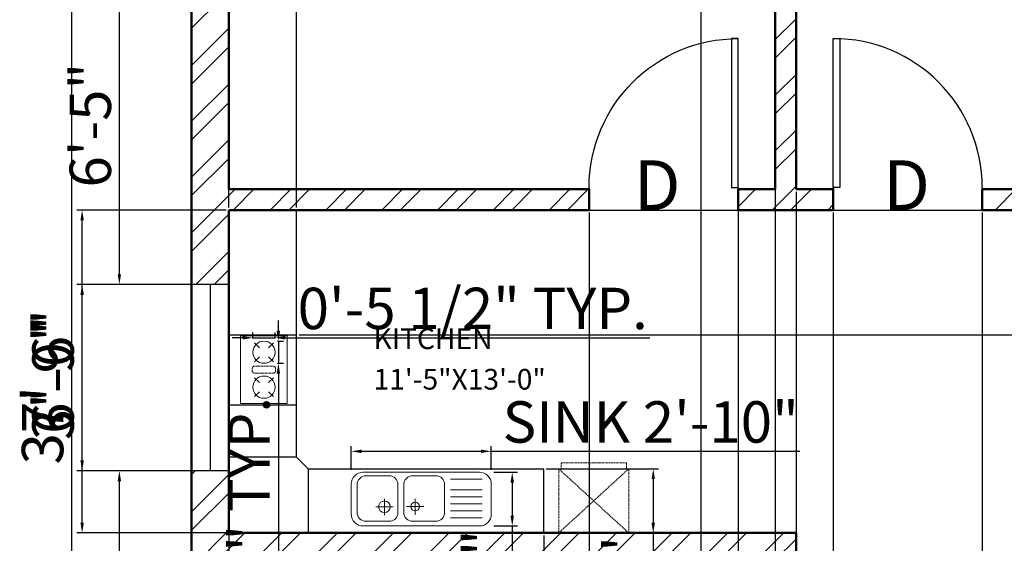
# Model space of a CAD drawing. Units: inches. Extents: x 3824 to 4289, y 1731 to 2259.
# Tile 3 of 5: x 3831 to 4069, y 1952 to 2079. Entities that reach past the tile are written whole.
import ezdxf

# ---------------------------------------------------------------- set-up
doc = ezdxf.new("R2010")
doc.units = ezdxf.units.IN
doc.linetypes.add('HIDDEN', pattern=[0.375, 0.25, -0.125])
for name, color, linetype, lineweight in [('A-ANNO-DIMS', 2, 'Continuous', 18), ('A-ANNO-TEXT', 2, 'Continuous', 18), ('A-AREA-IDEN', 2, 'Continuous', 18), ('A-EQPM', 9, 'Continuous', 18), ('A-EQPM-HIDN', 9, 'HIDDEN', 18), ('A-FLOR-CASE', 8, 'Continuous', 25), ('A-FLOR-FIXT', 9, 'Continuous', 18), ('A-FLOR-THRS', 8, 'Continuous', 18), ('DOOR', 6, 'Continuous', 25), ('WALL', 20, 'Continuous', 50), ('WINDOW', 4, 'Continuous', 25)]:
    doc.layers.add(name, color=color, linetype=linetype, lineweight=lineweight)
doc.layers.add('A-WALL-PATT', color=251, linetype='Continuous', lineweight=13, true_color=0x636466)
doc.styles.get("Standard").update_dxf_attribs({"font": 'arial.ttf'})
doc.dimstyles.new('ISO-25', dxfattribs={"dimtxt": 10, "dimasz": 2.5, "dimexe": 1.25, "dimexo": 0.625, "dimtad": 1, "dimdec": 1, "dimlunit": 3, "dimtxsty": 'Standard', "dimcen": 2.5, "dimadec": 0, "dimazin": 0, "dimtfac": 1, "dimtdec": 1, "dimtmove": 0, "dimatfit": 3, "dimfxl": 1, "dimarcsym": 0})

# ---------------------------------------------------------------- blocks, each defined once
blk = doc.blocks.new('*U2')
for p, q in [((0, 0), (0, -6)), ((40, 0), (40, -6))]:
    blk.add_line(p, q)
blk.add_lwpolyline([(0, 0), (0, 40), (1.75, 40), (1.75, 0)], close=True)
blk.add_arc((0, 0), 40, 0, 90)
blk = doc.blocks.new('SINK12RS')
for p, q in [((283, -292), (283, -153)), ((546, -293), (546, -154)), ((849, -130), (1120, -130)), ((209, -225), (359, -225)), ((472, -226), (622, -226)), ((849, -190), (1120, -190)), ((849, -250), (1120, -250)), ((849, -310), (1120, -310)), ((849, -370), (1120, -370)), ((849, -460), (1120, -460))]:
    blk.add_line(p, q)
for points in [[(99, -520), (1099, -520, 0.414214), (1199, -420), (1199, -160, 0.414214), (1099, -60), (99, -60, 0.414214), (-1, -160), (-1, -420, 0.414214)], [(124, -490), (324, -490, 0.414214), (399, -415), (399, -175, 0.414214), (324, -100), (124, -100, 0.414214), (49, -175), (49, -415, 0.414214)], [(524, -490, -0.414214), (449, -415), (449, -175, -0.414214), (524, -100), (724, -100, -0.414214), (799, -175), (799, -415, -0.414214), (724, -490)]]:
    blk.add_lwpolyline(points, format="xyb", close=True)
for centre, radius in [((283, -225), 50), ((546, -226), 37.5)]:
    blk.add_circle(centre, radius)
blk = doc.blocks.new('*D12')
at = {"layer": 'A-ANNO-DIMS', "color": 0, "lineweight": -2, "transparency": 16777216}
for p, q in [((3871.93, 2202.62), (3842.32, 2202.62)), ((3843.57, 2200.12), (3843.57, 1761.12)), ((3871.93, 1758.62), (3842.32, 1758.62))]:
    blk.add_line(p, q, dxfattribs=at)
at = {"layer": 'A-ANNO-DIMS', "color": 0, "transparency": 16777216}
for points in [[(3843.15, 2200.12), (3843.99, 2200.12), (3843.57, 2202.62)], [(3843.15, 1761.12), (3843.99, 1761.12), (3843.57, 1758.62)]]:
    blk.add_solid(points, dxfattribs=at)
at = {"layer": 'Defpoints', "color": 0, "transparency": 16777216}
for p in [(3872.55, 2202.62), (3843.57, 1758.62), (3872.55, 1758.62)]:
    blk.add_point(p, dxfattribs=at)
at = {"layer": 'A-ANNO-DIMS', "color": 0, "transparency": 16777216, "insert": (3837.84, 1980.62), "char_height": 10, "attachment_point": 5, "rotation": 90}
blk.add_mtext("37'", dxfattribs=at)
blk = doc.blocks.new('COOKTOP-BURNER')
for p, q in [((0.39, 4.97), (1.58, 3.77)), ((4.97, 4.97), (3.77, 3.77)), ((1.58, 1.58), (0.39, 0.39)), ((3.77, 1.58), (4.97, 0.39))]:
    blk.add_line(p, q)
blk.add_circle((2.68, 2.68), 2.68)
blk = doc.blocks.new('*D18')
at = {"layer": 'A-ANNO-DIMS', "color": 0, "lineweight": -2, "transparency": 16777216}
for p, q in [((3893.51, 2003.46), (3893.51, 2005.96)), ((3893.33, 2000.96), (3894.76, 2000.96)), ((3893.51, 2000.96), (3893.51, 1995.6)), ((3893.33, 1995.6), (3894.76, 1995.6)), ((3893.51, 1993.1), (3893.51, 1842.67))]:
    blk.add_line(p, q, dxfattribs=at)
at = {"layer": 'A-ANNO-DIMS', "color": 0, "transparency": 16777216}
for points in [[(3893.09, 2003.46), (3893.93, 2003.46), (3893.51, 2000.96)], [(3893.09, 1993.1), (3893.93, 1993.1), (3893.51, 1995.6)]]:
    blk.add_solid(points, dxfattribs=at)
at = {"layer": 'Defpoints', "color": 0, "transparency": 16777216}
for p in [(3892.71, 2000.96), (3892.71, 1995.6), (3893.51, 1995.6)]:
    blk.add_point(p, dxfattribs=at)
at = {"layer": 'A-ANNO-DIMS', "color": 0, "transparency": 16777216, "insert": (3887.71, 1916.64), "char_height": 10, "attachment_point": 5, "rotation": 90}
blk.add_mtext('BURNER 0\'-5 1/2" TYP.', dxfattribs=at)
blk = doc.blocks.new('*D19')
at = {"layer": 'A-ANNO-DIMS', "color": 0, "lineweight": -2, "transparency": 16777216}
for p, q in [((3887.35, 2001.58), (3887.35, 2003.01)), ((3892.71, 2001.58), (3892.71, 2003.01)), ((3884.85, 2001.76), (3882.35, 2001.76)), ((3887.35, 2001.76), (3892.71, 2001.76)), ((3895.21, 2001.76), (3983.21, 2001.76))]:
    blk.add_line(p, q, dxfattribs=at)
at = {"layer": 'A-ANNO-DIMS', "color": 0, "transparency": 16777216}
for points in [[(3884.85, 2002.17), (3884.85, 2001.34), (3887.35, 2001.76)], [(3895.21, 2002.17), (3895.21, 2001.34), (3892.71, 2001.76)]]:
    blk.add_solid(points, dxfattribs=at)
at = {"layer": 'Defpoints', "color": 0, "transparency": 16777216}
for p in [(3887.35, 2000.96), (3892.71, 2001.76), (3892.71, 2000.96)]:
    blk.add_point(p, dxfattribs=at)
at = {"layer": 'A-ANNO-DIMS', "color": 0, "transparency": 16777216, "insert": (3940.46, 2007.55), "char_height": 10, "attachment_point": 5}
blk.add_mtext('0\'-5 1/2" TYP.', dxfattribs=at)
blk = doc.blocks.new('*D22')
at = {"layer": 'A-ANNO-DIMS', "color": 0, "lineweight": -2, "transparency": 16777216}
for p, q in [((3911.13, 1969.89), (3911.13, 1975.59)), ((3913.63, 1974.34), (3942.43, 1974.34)), ((3944.93, 1969.89), (3944.93, 1975.59)), ((3944.93, 1974.34), (4019.47, 1974.34))]:
    blk.add_line(p, q, dxfattribs=at)
at = {"layer": 'A-ANNO-DIMS', "color": 0, "transparency": 16777216}
for points in [[(3913.63, 1974.75), (3913.63, 1973.92), (3911.13, 1974.34)], [(3942.43, 1974.75), (3942.43, 1973.92), (3944.93, 1974.34)]]:
    blk.add_solid(points, dxfattribs=at)
at = {"layer": 'Defpoints', "color": 0, "transparency": 16777216}
for p in [(3944.93, 1974.34), (3911.13, 1969.27), (3944.93, 1969.27)]:
    blk.add_point(p, dxfattribs=at)
at = {"layer": 'A-ANNO-DIMS', "color": 0, "transparency": 16777216, "insert": (3983.45, 1980.13), "char_height": 10, "attachment_point": 5}
blk.add_mtext('SINK 2\'-10"', dxfattribs=at)
blk = doc.blocks.new('*D23')
at = {"layer": 'A-ANNO-DIMS', "color": 0, "lineweight": -2, "transparency": 16777216}
for p, q in [((3945.56, 1969.27), (3951.25, 1969.27)), ((3950, 1966.77), (3950, 1958.81)), ((3945.56, 1956.31), (3951.25, 1956.31)), ((3950, 1956.31), (3950, 1926.92))]:
    blk.add_line(p, q, dxfattribs=at)
at = {"layer": 'A-ANNO-DIMS', "color": 0, "transparency": 16777216}
for points in [[(3949.58, 1966.77), (3950.42, 1966.77), (3950, 1969.27)], [(3949.58, 1958.81), (3950.42, 1958.81), (3950, 1956.31)]]:
    blk.add_solid(points, dxfattribs=at)
at = {"layer": 'Defpoints', "color": 0, "transparency": 16777216}
for p in [(3944.93, 1969.27), (3944.93, 1956.31), (3950, 1956.31)]:
    blk.add_point(p, dxfattribs=at)
at = {"layer": 'A-ANNO-DIMS', "color": 0, "transparency": 16777216, "insert": (3944.36, 1940.36), "char_height": 10, "attachment_point": 5, "rotation": 90}
blk.add_mtext('1\'-1"', dxfattribs=at)
blk = doc.blocks.new('*D28')
at = {"layer": 'A-ANNO-DIMS', "color": 0, "lineweight": -2, "transparency": 16777216}
for p, q in [((3880.93, 1969.62), (3853.85, 1969.62)), ((3855.1, 1904.12), (3855.1, 1967.12)), ((3880.93, 1901.62), (3853.85, 1901.62))]:
    blk.add_line(p, q, dxfattribs=at)
at = {"layer": 'A-ANNO-DIMS', "color": 0, "transparency": 16777216}
for points in [[(3854.69, 1967.12), (3855.52, 1967.12), (3855.1, 1969.62)], [(3854.69, 1904.12), (3855.52, 1904.12), (3855.1, 1901.62)]]:
    blk.add_solid(points, dxfattribs=at)
at = {"layer": 'Defpoints', "color": 0, "transparency": 16777216}
for p in [(3855.1, 1969.62), (3881.55, 1969.62), (3881.55, 1901.62)]:
    blk.add_point(p, dxfattribs=at)
at = {"layer": 'A-ANNO-DIMS', "color": 0, "transparency": 16777216, "insert": (3849.37, 1935.62), "char_height": 10, "attachment_point": 5, "rotation": 90}
blk.add_mtext('5\'-8"', dxfattribs=at)
blk = doc.blocks.new('*D29')
at = {"layer": 'A-ANNO-DIMS', "color": 0, "lineweight": -2, "transparency": 16777216}
for p, q in [((3871.93, 2014.62), (3844.85, 2014.62)), ((3846.1, 1972.12), (3846.1, 2012.12)), ((3871.93, 1969.62), (3844.85, 1969.62))]:
    blk.add_line(p, q, dxfattribs=at)
at = {"layer": 'A-ANNO-DIMS', "color": 0, "transparency": 16777216}
for points in [[(3845.69, 2012.12), (3846.52, 2012.12), (3846.1, 2014.62)], [(3845.69, 1972.12), (3846.52, 1972.12), (3846.1, 1969.62)]]:
    blk.add_solid(points, dxfattribs=at)
at = {"layer": 'Defpoints', "color": 0, "transparency": 16777216}
for p in [(3846.1, 2014.62), (3872.55, 2014.62), (3872.55, 1969.62)]:
    blk.add_point(p, dxfattribs=at)
at = {"layer": 'A-ANNO-DIMS', "color": 0, "transparency": 16777216, "insert": (3840.37, 1992.12), "char_height": 10, "attachment_point": 5, "rotation": 90}
blk.add_mtext('3\'-9"', dxfattribs=at)
blk = doc.blocks.new('*D30')
at = {"layer": 'A-ANNO-DIMS', "color": 0, "lineweight": -2, "transparency": 16777216}
for p, q in [((3880.93, 2091.62), (3853.85, 2091.62)), ((3855.1, 2017.12), (3855.1, 2089.12)), ((3880.93, 2014.62), (3853.85, 2014.62))]:
    blk.add_line(p, q, dxfattribs=at)
at = {"layer": 'A-ANNO-DIMS', "color": 0, "transparency": 16777216}
for points in [[(3854.69, 2089.12), (3855.52, 2089.12), (3855.1, 2091.62)], [(3854.69, 2017.12), (3855.52, 2017.12), (3855.1, 2014.62)]]:
    blk.add_solid(points, dxfattribs=at)
at = {"layer": 'Defpoints', "color": 0, "transparency": 16777216}
for p in [(3855.1, 2091.62), (3881.55, 2091.62), (3881.55, 2014.62)]:
    blk.add_point(p, dxfattribs=at)
at = {"layer": 'A-ANNO-DIMS', "color": 0, "transparency": 16777216, "insert": (3849.37, 2053.12), "char_height": 10, "attachment_point": 5, "rotation": 90}
blk.add_mtext('6\'-5"', dxfattribs=at)
blk = doc.blocks.new('*D42')
at = {"layer": 'A-ANNO-DIMS', "color": 0, "lineweight": -2, "transparency": 16777216}
for p, q in [((4004.55, 2036.99), (4004.55, 1730.92)), ((3968.55, 2031.99), (3968.55, 1730.92)), ((3971.05, 1732.17), (4002.05, 1732.17))]:
    blk.add_line(p, q, dxfattribs=at)
at = {"layer": 'A-ANNO-DIMS', "color": 0, "transparency": 16777216}
for points in [[(3971.05, 1732.59), (3971.05, 1731.75), (3968.55, 1732.17)], [(4002.05, 1732.59), (4002.05, 1731.75), (4004.55, 1732.17)]]:
    blk.add_solid(points, dxfattribs=at)
at = {"layer": 'Defpoints', "color": 0, "transparency": 16777216}
for p in [(4004.55, 2037.62), (3968.55, 2032.62), (4004.55, 1732.17)]:
    blk.add_point(p, dxfattribs=at)
at = {"layer": 'A-ANNO-DIMS', "color": 0, "transparency": 16777216, "insert": (3986.55, 1737.9), "char_height": 10, "attachment_point": 5}
blk.add_mtext('3\'-0"', dxfattribs=at)
blk = doc.blocks.new('*D43')
at = {"layer": 'A-ANNO-DIMS', "color": 0, "lineweight": -2, "transparency": 16777216}
for p, q in [((4004.55, 2036.99), (4004.55, 1730.92)), ((4013.55, 2036.99), (4013.55, 1730.92)), ((4007.05, 1732.17), (4011.05, 1732.17)), ((4013.55, 1732.17), (4043.88, 1732.17))]:
    blk.add_line(p, q, dxfattribs=at)
at = {"layer": 'A-ANNO-DIMS', "color": 0, "transparency": 16777216}
for points in [[(4007.05, 1732.59), (4007.05, 1731.75), (4004.55, 1732.17)], [(4011.05, 1732.59), (4011.05, 1731.75), (4013.55, 1732.17)]]:
    blk.add_solid(points, dxfattribs=at)
at = {"layer": 'Defpoints', "color": 0, "transparency": 16777216}
for p in [(4004.55, 2037.62), (4013.55, 2037.62), (4013.55, 1732.17)]:
    blk.add_point(p, dxfattribs=at)
at = {"layer": 'A-ANNO-DIMS', "color": 0, "transparency": 16777216, "insert": (4029.97, 1737.9), "char_height": 10, "attachment_point": 5}
blk.add_mtext('0\'-9"', dxfattribs=at)
blk = doc.blocks.new('*D44')
at = {"layer": 'A-ANNO-DIMS', "color": 0, "lineweight": -2, "transparency": 16777216}
for p, q in [((4018.55, 2036.99), (4018.55, 1730.92)), ((4027.55, 2031.99), (4027.55, 1730.92)), ((4021.05, 1732.17), (4025.05, 1732.17)), ((4027.55, 1732.17), (4057.88, 1732.17))]:
    blk.add_line(p, q, dxfattribs=at)
at = {"layer": 'A-ANNO-DIMS', "color": 0, "transparency": 16777216}
for points in [[(4021.05, 1732.59), (4021.05, 1731.75), (4018.55, 1732.17)], [(4025.05, 1732.59), (4025.05, 1731.75), (4027.55, 1732.17)]]:
    blk.add_solid(points, dxfattribs=at)
at = {"layer": 'Defpoints', "color": 0, "transparency": 16777216}
for p in [(4018.55, 2037.62), (4027.55, 2032.62), (4027.55, 1732.17)]:
    blk.add_point(p, dxfattribs=at)
at = {"layer": 'A-ANNO-DIMS', "color": 0, "transparency": 16777216, "insert": (4043.97, 1737.9), "char_height": 10, "attachment_point": 5}
blk.add_mtext('0\'-9"', dxfattribs=at)
blk = doc.blocks.new('*D45')
at = {"layer": 'A-ANNO-DIMS', "color": 0, "lineweight": -2, "transparency": 16777216}
for p, q in [((4027.55, 2031.99), (4027.55, 1730.92)), ((4063.55, 2031.99), (4063.55, 1730.92)), ((4030.05, 1732.17), (4061.05, 1732.17))]:
    blk.add_line(p, q, dxfattribs=at)
at = {"layer": 'A-ANNO-DIMS', "color": 0, "transparency": 16777216}
for points in [[(4030.05, 1732.59), (4030.05, 1731.75), (4027.55, 1732.17)], [(4061.05, 1732.59), (4061.05, 1731.75), (4063.55, 1732.17)]]:
    blk.add_solid(points, dxfattribs=at)
at = {"layer": 'Defpoints', "color": 0, "transparency": 16777216}
for p in [(4027.55, 2032.62), (4063.55, 2032.62), (4063.55, 1732.17)]:
    blk.add_point(p, dxfattribs=at)
at = {"layer": 'A-ANNO-DIMS', "color": 0, "transparency": 16777216, "insert": (4045.55, 1737.9), "char_height": 10, "attachment_point": 5}
blk.add_mtext('3\'-0"', dxfattribs=at)
blk = doc.blocks.new('*D56')
at = {"layer": 'A-ANNO-DIMS', "color": 0, "lineweight": -2, "transparency": 16777216}
for p, q in [((3995.55, 2120.99), (3995.55, 1730.92)), ((4013.55, 2120.99), (4013.55, 1730.92)), ((3998.05, 1732.17), (4011.05, 1732.17)), ((4013.55, 1732.17), (4042.94, 1732.17))]:
    blk.add_line(p, q, dxfattribs=at)
at = {"layer": 'A-ANNO-DIMS', "color": 0, "transparency": 16777216}
for points in [[(3998.05, 1732.59), (3998.05, 1731.75), (3995.55, 1732.17)], [(4011.05, 1732.59), (4011.05, 1731.75), (4013.55, 1732.17)]]:
    blk.add_solid(points, dxfattribs=at)
at = {"layer": 'Defpoints', "color": 0, "transparency": 16777216}
for p in [(3995.55, 2121.62), (4013.55, 2121.62), (4013.55, 1732.17)]:
    blk.add_point(p, dxfattribs=at)
at = {"layer": 'A-ANNO-DIMS', "color": 0, "transparency": 16777216, "insert": (4029.5, 1737.9), "char_height": 10, "attachment_point": 5}
blk.add_mtext('1\'-6"', dxfattribs=at)
blk = doc.blocks.new('*D58')
at = {"layer": 'A-ANNO-DIMS', "color": 0, "lineweight": -2, "transparency": 16777216}
for p, q in [((3881.55, 1953.99), (3881.55, 1730.92)), ((3957.61, 1953.99), (3957.61, 1730.92)), ((3884.05, 1732.17), (3955.11, 1732.17))]:
    blk.add_line(p, q, dxfattribs=at)
at = {"layer": 'A-ANNO-DIMS', "color": 0, "transparency": 16777216}
for points in [[(3884.05, 1732.59), (3884.05, 1731.75), (3881.55, 1732.17)], [(3955.11, 1732.59), (3955.11, 1731.75), (3957.61, 1732.17)]]:
    blk.add_solid(points, dxfattribs=at)
at = {"layer": 'Defpoints', "color": 0, "transparency": 16777216}
for p in [(3881.55, 1954.62), (3957.61, 1954.62), (3957.61, 1732.17)]:
    blk.add_point(p, dxfattribs=at)
at = {"layer": 'A-ANNO-DIMS', "color": 0, "transparency": 16777216, "insert": (3919.58, 1737.9), "char_height": 10, "attachment_point": 5}
blk.add_mtext('6\'-4"', dxfattribs=at)
blk = doc.blocks.new('*D59')
at = {"layer": 'A-ANNO-DIMS', "color": 0, "lineweight": -2, "transparency": 16777216}
for p, q in [((3881.55, 2033.24), (3881.55, 2230.32)), ((3884.05, 2229.07), (3895.39, 2229.07)), ((3897.89, 2033.24), (3897.89, 2230.32)), ((3897.89, 2229.07), (3950.58, 2229.07))]:
    blk.add_line(p, q, dxfattribs=at)
at = {"layer": 'A-ANNO-DIMS', "color": 0, "transparency": 16777216}
for points in [[(3884.05, 2229.49), (3884.05, 2228.65), (3881.55, 2229.07)], [(3895.39, 2229.49), (3895.39, 2228.65), (3897.89, 2229.07)]]:
    blk.add_solid(points, dxfattribs=at)
at = {"layer": 'Defpoints', "color": 0, "transparency": 16777216}
for p in [(3897.89, 2229.07), (3881.55, 2032.62), (3897.89, 2032.62)]:
    blk.add_point(p, dxfattribs=at)
at = {"layer": 'A-ANNO-DIMS', "color": 0, "transparency": 16777216, "insert": (3925.49, 2234.86), "char_height": 10, "attachment_point": 5}
blk.add_mtext('1\'-4 1/2"', dxfattribs=at)
blk = doc.blocks.new('*D60')
at = {"layer": 'A-ANNO-DIMS', "color": 0, "lineweight": -2, "transparency": 16777216}
for p, q in [((3880.93, 2032.62), (3844.85, 2032.62)), ((3846.1, 1957.12), (3846.1, 2030.12)), ((3880.93, 1954.62), (3844.85, 1954.62))]:
    blk.add_line(p, q, dxfattribs=at)
at = {"layer": 'A-ANNO-DIMS', "color": 0, "transparency": 16777216}
for points in [[(3845.69, 2030.12), (3846.52, 2030.12), (3846.1, 2032.62)], [(3845.69, 1957.12), (3846.52, 1957.12), (3846.1, 1954.62)]]:
    blk.add_solid(points, dxfattribs=at)
at = {"layer": 'Defpoints', "color": 0, "transparency": 16777216}
for p in [(3846.1, 2032.62), (3881.55, 2032.62), (3881.55, 1954.62)]:
    blk.add_point(p, dxfattribs=at)
at = {"layer": 'A-ANNO-DIMS', "color": 0, "transparency": 16777216, "insert": (3840.37, 1993.62), "char_height": 10, "attachment_point": 5, "rotation": 90}
blk.add_mtext('6\'-6"', dxfattribs=at)
blk = doc.blocks.new('*D61')
at = {"layer": 'A-ANNO-DIMS', "color": 0, "lineweight": -2, "transparency": 16777216}
for p, q in [((3958.23, 1970.11), (3985.31, 1970.11)), ((3984.06, 1967.61), (3984.06, 1957.12)), ((3958.23, 1954.62), (3985.31, 1954.62)), ((3984.06, 1954.62), (3984.06, 1901.93))]:
    blk.add_line(p, q, dxfattribs=at)
at = {"layer": 'A-ANNO-DIMS', "color": 0, "transparency": 16777216}
for points in [[(3983.64, 1967.61), (3984.47, 1967.61), (3984.06, 1970.11)], [(3983.64, 1957.12), (3984.47, 1957.12), (3984.06, 1954.62)]]:
    blk.add_solid(points, dxfattribs=at)
at = {"layer": 'Defpoints', "color": 0, "transparency": 16777216}
for p in [(3957.61, 1970.11), (3957.61, 1954.62), (3984.06, 1954.62)]:
    blk.add_point(p, dxfattribs=at)
at = {"layer": 'A-ANNO-DIMS', "color": 0, "transparency": 16777216, "insert": (3978.26, 1927.02), "char_height": 10, "attachment_point": 5, "rotation": 90}
blk.add_mtext('1\'-3 1/2"', dxfattribs=at)
blk = doc.blocks.new('*D62')
at = {"layer": 'A-ANNO-DIMS', "color": 0, "lineweight": -2, "transparency": 16777216}
for p, q in [((3898.51, 2032.62), (4188.25, 2032.62)), ((4187, 2005), (4187, 2030.12)), ((3898.51, 2002.5), (4188.25, 2002.5))]:
    blk.add_line(p, q, dxfattribs=at)
at = {"layer": 'A-ANNO-DIMS', "color": 0, "transparency": 16777216}
for points in [[(4186.59, 2030.12), (4187.42, 2030.12), (4187, 2032.62)], [(4186.59, 2005), (4187.42, 2005), (4187, 2002.5)]]:
    blk.add_solid(points, dxfattribs=at)
at = {"layer": 'Defpoints', "color": 0, "transparency": 16777216}
for p in [(3897.89, 2032.62), (4187, 2032.62), (3897.89, 2002.5)]:
    blk.add_point(p, dxfattribs=at)
at = {"layer": 'A-ANNO-DIMS', "color": 0, "transparency": 16777216, "insert": (4181.27, 2017.56), "char_height": 10, "attachment_point": 5, "rotation": 90}
blk.add_mtext('2\'-6"', dxfattribs=at)

msp = doc.modelspace()

# ---------------------------------------------------------------- hatches: boundary and pattern name
at = {"layer": 'A-WALL-PATT'}
h = msp.add_hatch(dxfattribs=at)
h.set_pattern_fill('ANSI32', color=256)
h.paths.add_polyline_path([(4160.55, 2202.62), (3872.55, 2202.62), (3872.55, 2139.62), (3881.55, 2139.62), (3881.55, 2193.62), (4013.55, 2193.62), (4013.55, 2037.62), (4004.55, 2037.62), (4004.55, 2032.62), (4027.55, 2032.62), (4027.55, 2037.62), (4018.55, 2037.62), (4018.55, 2193.62), (4036.55, 2193.62), (4151.55, 2193.62), (4151.55, 2139.62), (4160.55, 2139.62)])
h = msp.add_hatch(dxfattribs=at)
h.set_pattern_fill('ANSI32', color=256)
h.paths.add_polyline_path([(3881.55, 2091.62), (3872.55, 2091.62), (3872.55, 2014.62), (3881.55, 2014.62), (3881.55, 2032.62), (3897.89, 2032.62), (3968.55, 2032.62), (3968.55, 2037.62), (3881.55, 2037.62)])
h = msp.add_hatch(dxfattribs=at)
h.set_pattern_fill('ANSI32', color=256)
h.paths.add_polyline_path([(4160.55, 2091.62), (4151.55, 2091.62), (4151.55, 2037.62), (4063.55, 2037.62), (4063.55, 2032.62), (4151.55, 2032.62), (4151.55, 2008.62), (4160.55, 2008.62)])
h = msp.add_hatch(dxfattribs=at)
h.set_pattern_fill('ANSI32', color=256)
h.paths.add_polyline_path([(4018.55, 1954.62), (3881.55, 1954.62), (3881.55, 1969.62), (3872.55, 1969.62), (3872.55, 1901.62), (3881.53, 1901.62), (3881.53, 1903.2, -0.148069), (3880.67, 1906.03, -0.148069), (3881.53, 1908.87), (3881.53, 1910.29), (3881.55, 1949.62), (4013.55, 1949.62), (4013.55, 1940.62), (4018.55, 1940.62)])

# ---------------------------------------------------------------- linework, layer by layer
at = {"layer": 'A-EQPM'}
for p, q in [((3884.37, 2002.22), (3895.64, 2002.22)), ((3884.37, 1985.89), (3884.37, 2002.22)), ((3895.64, 2002.22), (3895.64, 1985.89)), ((3895.64, 1985.89), (3884.37, 1985.89))]:
    msp.add_line(p, q, dxfattribs=at)
at = {"layer": 'A-EQPM-HIDN'}
for p, q in [((3887.19, 1993.77), (3887.19, 1994.34)), ((3887.75, 1994.9), (3892.26, 1994.9)), ((3892.26, 1993.21), (3887.75, 1993.21)), ((3892.82, 1994.34), (3892.82, 1993.77)), ((3978.13, 1970.11), (3961.23, 1970.11)), ((3961.23, 1970.11), (3978.13, 1954.62)), ((3978.13, 1970.11), (3961.23, 1954.62)), ((3961.23, 1970.11), (3961.23, 1954.62)), ((3978.13, 1954.62), (3978.13, 1970.11)), ((3961.23, 1954.62), (3978.13, 1954.62))]:
    msp.add_line(p, q, dxfattribs=at)
msp.add_lwpolyline([(3961.79, 1970.11), (3961.79, 1971.52), (3977.57, 1971.52), (3977.57, 1970.11)], dxfattribs=at)
for centre, start, end in [((3887.75, 1994.34), 90, 180), ((3887.75, 1993.77), 180, 270), ((3892.26, 1994.34), 0, 90), ((3892.26, 1993.77), 270, 0)]:
    msp.add_arc(centre, 0.563, start, end, dxfattribs=at)
at = {"layer": 'A-FLOR-CASE'}
for p, q in [((3881.55, 2032.62), (3897.89, 2032.62)), ((3881.55, 1954.62), (3881.55, 2032.62)), ((3897.89, 1972.93), (3897.89, 2032.62)), ((3881.55, 2002.5), (3897.89, 2002.5)), ((3881.55, 1985.6), (3897.89, 1985.6)), ((3897.89, 1972.93), (3881.55, 1972.93)), ((3897.89, 1972.93), (3900.71, 1970.11)), ((3881.55, 1954.62), (3881.55, 1970.11)), ((3900.71, 1970.11), (3957.61, 1970.11)), ((3900.71, 1970.11), (3900.71, 1954.62)), ((3957.61, 1954.62), (3957.61, 1970.11)), ((3881.55, 1954.62), (3957.61, 1954.62))]:
    msp.add_line(p, q, dxfattribs=at)
at = {"layer": 'A-FLOR-THRS'}
for p, q in [((3968.55, 2032.62), (4004.55, 2032.62)), ((4027.55, 2032.62), (4063.55, 2032.62))]:
    msp.add_line(p, q, dxfattribs=at)
at = {"layer": 'WALL'}
for p, q in [((3872.55, 2202.62), (3872.55, 1758.62)), ((3881.55, 2193.62), (3881.55, 2037.62)), ((4013.55, 2193.62), (4013.55, 2037.62)), ((4018.55, 2193.62), (4018.55, 2037.62)), ((3881.55, 2037.62), (3968.55, 2037.62)), ((3968.55, 2037.62), (3968.55, 2032.62)), ((4004.55, 2037.62), (4004.55, 2032.62)), ((4004.55, 2037.62), (4013.55, 2037.62)), ((4018.55, 2037.62), (4027.55, 2037.62)), ((4027.55, 2037.62), (4027.55, 2032.62)), ((4063.55, 2037.62), (4063.55, 2032.62)), ((4063.55, 2037.62), (4151.55, 2037.62)), ((3881.55, 2032.62), (3968.55, 2032.62)), ((3881.55, 2032.62), (3881.55, 1954.62)), ((4004.55, 2032.62), (4027.55, 2032.62)), ((4063.55, 2032.62), (4151.55, 2032.62)), ((3881.55, 1954.62), (4018.55, 1954.62)), ((4018.55, 1954.62), (4018.55, 1940.62))]:
    msp.add_line(p, q, dxfattribs=at)
at = {"layer": 'WINDOW'}
for p, q in [((3881.55, 2014.62), (3872.55, 2014.62)), ((3877.05, 2014.62), (3877.05, 1969.62)), ((3881.55, 1969.62), (3872.55, 1969.62))]:
    msp.add_line(p, q, dxfattribs=at)

# ---------------------------------------------------------------- block references
at = {"layer": 'A-EQPM', "rotation": 270.0000000000142}
msp.add_blockref('COOKTOP-BURNER', (3887.35, 2000.95), dxfattribs=at)
at = {"layer": 'A-EQPM'}
msp.add_blockref('COOKTOP-BURNER', (3887.35, 1987.15), dxfattribs=at)
at = {"layer": 'A-FLOR-FIXT', "xscale": -0.0281680997421484, "yscale": 0.0281680997421484, "zscale": 0.0281680997421484, "rotation": 180}
msp.add_blockref('SINK12RS', (3911.16, 1954.62), dxfattribs=at)
at = {"layer": 'DOOR', "yscale": 0.9, "zscale": 0.9}
for p, xscale in [((4004.55, 2038.02), -0.9), ((4027.55, 2038.02), 0.9)]:
    msp.add_blockref('*U2', p, dxfattribs=dict(at, xscale=xscale))

# ---------------------------------------------------------------- texts
at = {"layer": 'A-ANNO-TEXT'}
for p in [(3979.38, 2032.62), (4039.62, 2032.62)]:
    msp.add_text('D', height=12, dxfattribs=at).set_placement(p)
at = {"layer": 'A-AREA-IDEN'}
for s, p in [('KITCHEN', (3916.49, 1999.02)), ('11\'-5"X13\'-0"', (3916.49, 1989.24))]:
    msp.add_text(s, height=5, dxfattribs=at).set_placement(p)

# ---------------------------------------------------------------- dimensions: what is measured, and where the dimension line sits
at = {"layer": 'A-ANNO-DIMS'}
for base, p1, p2, picture, middle in [((3897.89, 2229.07), (3881.55, 2032.62), (3897.89, 2032.62), '*D59', (3925.49, 2234.86)), ((4013.55, 1732.17), (3995.55, 2121.62), (4013.55, 2121.62), '*D56', (4029.5, 1737.9)), ((4004.55, 1732.17), (3968.55, 2032.62), (4004.55, 2037.62), '*D42', (3986.55, 1737.9)), ((4013.55, 1732.17), (4004.55, 2037.62), (4013.55, 2037.62), '*D43', (4029.97, 1737.9)), ((4027.55, 1732.17), (4018.55, 2037.62), (4027.55, 2032.62), '*D44', (4043.97, 1737.9)), ((4063.55, 1732.17), (4027.55, 2032.62), (4063.55, 2032.62), '*D45', (4045.55, 1737.9)), ((3957.61, 1732.17), (3881.55, 1954.62), (3957.61, 1954.62), '*D58', (3919.58, 1737.9))]:
    dim = msp.add_linear_dim(base=base, p1=p1, p2=p2, dimstyle='ISO-25', override={"dimdec": 1, "dimlfac": 1, "dimrnd": 0, "dimzin": 1, "dimdsep": 46, "dimlunit": 4, "dimfrac": 2}, dxfattribs=at)
    dim.commit()
    dim.dimension.update_dxf_attribs({"geometry": picture, "text_midpoint": middle})
for base, p1, p2, angle, override, picture, middle in [((3843.57, 1758.62), (3872.55, 2202.62), (3872.55, 1758.62), 90, {"dimclrd": 0, "dimclre": 0, "dimclrt": 0}, '*D12', (3837.84, 1980.62)), ((3855.1, 2091.62), (3881.55, 2014.62), (3881.55, 2091.62), 90, {"dimdec": 1, "dimlfac": 1, "dimrnd": 0, "dimzin": 1, "dimdsep": 46, "dimlunit": 4, "dimfrac": 2}, '*D30', (3849.37, 2053.12)), ((3846.1, 2032.62), (3881.55, 1954.62), (3881.55, 2032.62), 90, {"dimdec": 1, "dimlfac": 1, "dimrnd": 0, "dimzin": 1, "dimdsep": 46, "dimlunit": 4, "dimfrac": 2}, '*D60', (3840.37, 1993.62)), ((4187, 2032.62), (3897.89, 2002.5), (3897.89, 2032.62), 90, {"dimdec": 1, "dimlfac": 1, "dimrnd": 0, "dimzin": 1, "dimdsep": 46, "dimlunit": 4, "dimfrac": 2}, '*D62', (4181.27, 2017.56)), ((3846.1, 2014.62), (3872.55, 1969.62), (3872.55, 2014.62), 90, {"dimdec": 1, "dimlfac": 1, "dimrnd": 0, "dimzin": 1, "dimdsep": 46, "dimlunit": 4, "dimfrac": 2}, '*D29', (3840.37, 1992.12)), ((3855.1, 1969.62), (3881.55, 1901.62), (3881.55, 1969.62), 90, {"dimdec": 1, "dimlfac": 1, "dimrnd": 0, "dimzin": 1, "dimdsep": 46, "dimlunit": 4, "dimfrac": 2}, '*D28', (3849.37, 1935.62)), ((3984.06, 1954.62), (3957.61, 1970.11), (3957.61, 1954.62), 270, {"dimdec": 1, "dimlfac": 1, "dimrnd": 0, "dimzin": 1, "dimdsep": 46, "dimlunit": 4, "dimfrac": 2}, '*D61', (3978.26, 1927.02)), ((3950, 1956.31), (3944.93, 1969.27), (3944.93, 1956.31), 270, {"dimdec": 1, "dimlfac": 1, "dimrnd": 0, "dimzin": 1, "dimdsep": 46, "dimlunit": 4, "dimfrac": 2}, '*D23', (3944.36, 1940.36))]:
    dim = msp.add_linear_dim(base=base, p1=p1, p2=p2, angle=angle, dimstyle='ISO-25', override=override, dxfattribs=at)
    dim.commit()
    dim.dimension.update_dxf_attribs({"geometry": picture, "text_midpoint": middle})
for base, p1, p2, angle, text, picture, middle in [((3892.71, 2001.76), (3887.35, 2000.96), (3892.71, 2000.96), 0, '<> TYP.', '*D19', (3940.46, 2007.55)), ((3893.51, 1995.6), (3892.71, 2000.96), (3892.71, 1995.6), 270, 'BURNER <> TYP.', '*D18', (3887.71, 1916.64))]:
    dim = msp.add_linear_dim(base=base, p1=p1, p2=p2, angle=angle, text=text, dimstyle='ISO-25', override={"dimdec": 1, "dimlfac": 1, "dimrnd": 0, "dimzin": 1, "dimdsep": 46, "dimlunit": 4, "dimfrac": 2}, dxfattribs=at)
    dim.commit()
    dim.dimension.update_dxf_attribs({"geometry": picture, "text_midpoint": middle})
dim = msp.add_linear_dim(base=(3944.93, 1974.34), p1=(3911.13, 1969.27), p2=(3944.93, 1969.27), text='SINK <>', dimstyle='ISO-25', override={"dimdec": 1, "dimlfac": 1, "dimrnd": 0, "dimzin": 1, "dimdsep": 46, "dimlunit": 4, "dimfrac": 2}, dxfattribs=at)
dim.commit()
dim.dimension.update_dxf_attribs({"geometry": '*D22', "text_midpoint": (3983.45, 1980.13)})

doc.saveas('drawing.dxf')
